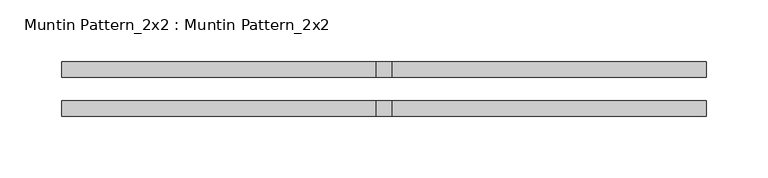
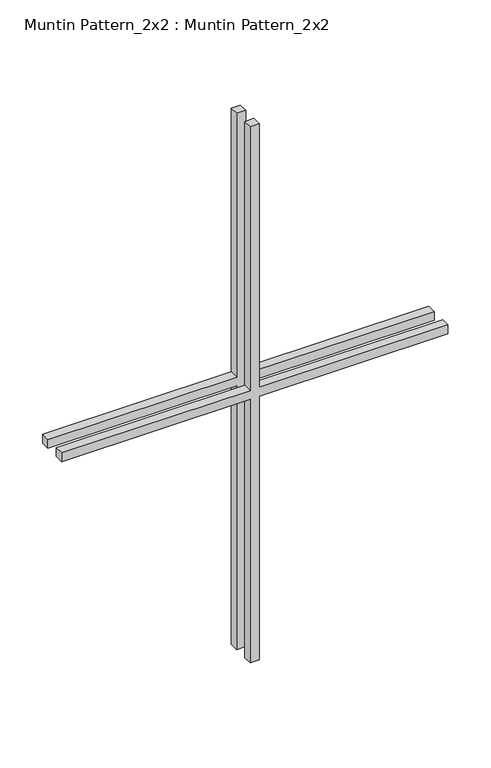
"""IFC4 building model written with IfcOpenShell, lengths in millimetres: proxy geometry, Muntin Pattern_2x2 : Muntin Pattern_2x2."""

from ifc_helpers import new_model, si_unit, frame, origin, place, context, project, spatial, polyline, outline, extrude, source, transform, mapped, element, save


def muntin_pattern_2x2_muntin_pattern_2x2_0ac132d2(model_context):
    return source(origin(), model_context, "Body", "SweptSolid", [
        extrude(outline(polyline([(390.525, -6.35), (390.525, -261.9375), (377.825, -261.9375), (377.825, -6.35), (0.0, -6.35), (0.0, 6.35), (377.825, 6.35), (377.825, 261.9375), (390.525, 261.9375), (390.525, 6.35), (768.35, 6.35), (768.35, -6.35), (390.525, -6.35)])), frame((0.0, 9.525, 0.0), z_axis=(0.0, 1.0, 0.0), x_axis=(0.0, 0.0, 1.0)), (0.0, 0.0, 1.0), 12.7),
        extrude(outline(polyline([(390.525, -6.35), (390.525, -261.9375), (377.825, -261.9375), (377.825, -6.35), (0.0, -6.35), (0.0, 6.35), (377.825, 6.35), (377.825, 261.9375), (390.525, 261.9375), (390.525, 6.35), (768.35, 6.35), (768.35, -6.35), (390.525, -6.35)])), frame((0.0, -22.225, 0.0), z_axis=(0.0, 1.0, 0.0), x_axis=(0.0, 0.0, 1.0)), (0.0, 0.0, 1.0), 12.7),
    ])


if __name__ == "__main__":
    model = new_model("IFC4")
    model_context = context("Model", 3, world=origin())
    ifc_project = project(units=[si_unit("LENGTHUNIT", "METRE", prefix="MILLI")], contexts=[model_context])
    site = spatial("IfcSite", under=ifc_project)
    building = spatial("IfcBuilding", under=site)
    placement = place(None, origin())
    muntin_pattern_2x2_muntin_pattern_2x2_shape = muntin_pattern_2x2_muntin_pattern_2x2_0ac132d2(model_context)
    element("IfcBuildingElementProxy", 1, Name="Muntin Pattern_2x2 : Muntin Pattern_2x2", ObjectType="Muntin Pattern_2x2 : Muntin Pattern_2x2", at=placement, inside=building, context=model_context, shape_type="MappedRepresentation", body=[
        mapped(muntin_pattern_2x2_muntin_pattern_2x2_shape, transform((0.0, 0.0, 0.0), x_axis=(1.0, 0.0, 0.0), y_axis=(0.0, 1.0, 0.0), z_axis=(0.0, 0.0, 1.0))),
    ])
    save(model, "model.ifc")

# Revit data of these elements
# Type "Muntin Pattern_2x2 : Muntin Pattern_2x2"
#   Width [instance default] = 4' - 0"
#   Thickness = 0' - 0 1/2"
#   Height [instance default] = 4' - 0"
#   Distance = 0' - 0 3/4"
#   Interior Material [instance default] = none
#   Exterior Material [instance default] = none
#   Default Elevation = 0
# Element 1 (IfcBuildingElementProxy, "Muntin Pattern_2x2 : Muntin Pattern_2x2")
#   Width = 1' - 8 5/8"
#   Height = 2' - 6 1/4"
#   Interior Material = Wood - Stained
#   Exterior Material = Clad - White
#   Materials on its faces: "Clad - White", "Wood - Stained"
# Materials
#   "Clad - White": class "Wood", colour RGB 242 242 238, transparency 0, Cost = 0
#   "Wood - Stained": class "Wood", colour RGB 224 178 126, transparency 0, Cost = 0
